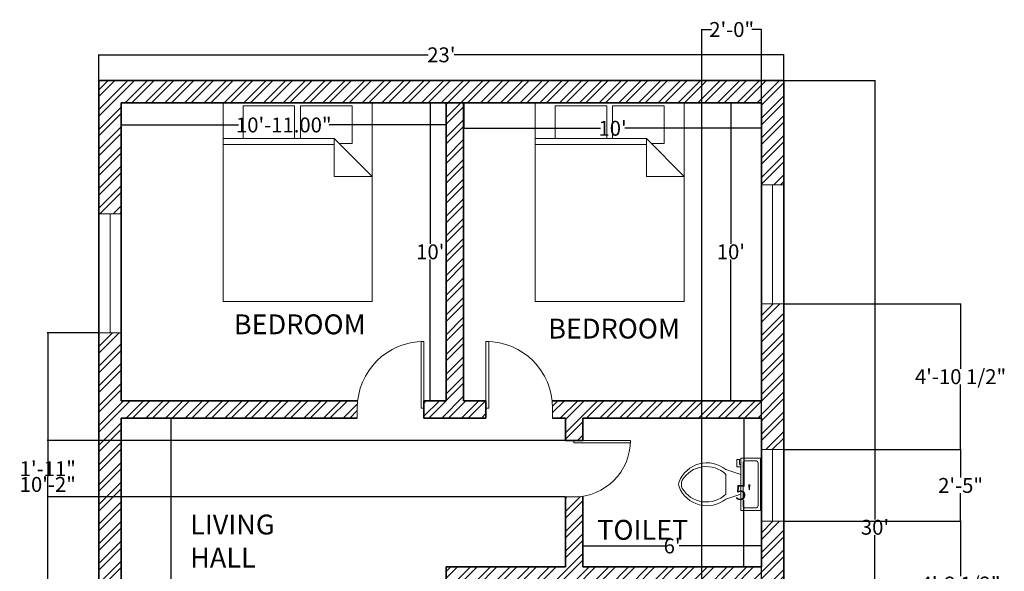
# Model space of a CAD drawing. Units: inches. Extents: x -20 to 887, y -143 to 410.
# Tile 3 of 5: x -15 to 381, y 180 to 403. Entities that reach past the tile are written whole.
import ezdxf

# ---------------------------------------------------------------- set-up
doc = ezdxf.new("R2010")
doc.units = ezdxf.units.IN
doc.header["$MEASUREMENT"] = 0
for name, color, linetype, lineweight in [('A-ANNO-DIMS', 2, 'Continuous', 18), ('A-AREA-IDEN', 7, 'Continuous', 25), ('A-DOOR', 3, 'Continuous', 18), ('A-FLOR-FIXT', 9, 'Continuous', 18), ('A-FURN', 8, 'Continuous', 18), ('A-GLAZ', 4, 'Continuous', 18), ('A-WALL', 7, 'Continuous', 35), ('A-WALL-PATT', 8, 'Continuous', 13)]:
    doc.layers.add(name, color=color, linetype=linetype, lineweight=lineweight)
doc.styles.get("Standard").update_dxf_attribs({"font": 'arial.ttf'})
doc.dimstyles.get("Standard").update_dxf_attribs({"dimtxt": 6, "dimasz": 0.18, "dimexe": 0.18, "dimexo": 0.0625, "dimgap": 0.09, "dimtad": 0, "dimtih": 1, "dimtoh": 1, "dimzin": 0, "dimdsep": 46, "dimlunit": 3, "dimtxsty": 'Standard', "dimcen": 0.09, "dimadec": 0, "dimazin": 0, "dimtfac": 1, "dimtofl": 0, "dimtmove": 0, "dimatfit": 3, "dimfxl": 1, "dimtolj": 1, "dimtzin": 0, "dimarcsym": 0})

# ---------------------------------------------------------------- blocks, each defined once
blk = doc.blocks.new('*U2')
for p, q in [((0, 0), (0, -6)), ((40, 0), (40, -6))]:
    blk.add_line(p, q)
blk.add_lwpolyline([(0, 0), (0, 40), (1.75, 40), (1.75, 0)], close=True)
blk.add_arc((0, 0), 40, 0, 90)
blk = doc.blocks.new('*U6')
for p, q in [((9.5, -6), (9.5, -2)), ((-10, -8.5), (-8, -8.5)), ((-10, -9.5), (-10, -8.5)), ((-7, -9.5), (-10, -9.5)), ((-8, -8.5), (-8, -8)), ((-7, -8), (-7, -9.5)), ((-4, -8), (-6, -14)), ((4, -8), (6, -14)), ((4, -14), (-4, -14))]:
    blk.add_line(p, q)
blk.add_lwpolyline([(10.5, -8), (10.5, 0), (-10.5, 0), (-10.5, -8)], close=True)
for points in [[(-9.5, -2), (-9.5, -6)], [(8.5, -1), (-8.5, -1)], [(-8.5, -7), (8.5, -7)]]:
    blk.add_lwpolyline(points)
for centre, radius, start, end in [((-8.62, -1.88), 0.884, 81.8699, 188.1301), ((8.62, -1.88), 0.884, 351.8699, 98.1301), ((-8.62, -6.12), 0.884, 171.8699, 278.1301), ((8.62, -6.12), 0.884, 261.8699, 8.1301), ((3.52, -21.58), 12.17, 141.4691, 247.9714), ((4.2, -21.82), 11.33, 136.3677, 238.9468), ((-3.52, -21.58), 12.17, 292.0284, 38.5307), ((-4.2, -21.82), 11.33, 301.053, 43.6321), ((0, -27.88), 4, 245.7318, 294.2682), ((0, -29), 4, 254.8605, 285.1395)]:
    blk.add_arc(centre, radius, start, end)
blk = doc.blocks.new('Bed - Queen')
for p, q in [((0, -80.00003), (0, 0)), ((0, 0), (59.99999, 0)), ((59.99999, 0), (59.99999, -80.00003)), ((7.99999, -1.2), (28.79998, -1.2)), ((7.99999, -14.4), (7.99999, -1.2)), ((28.79998, -1.2), (28.79998, -14.4)), ((31.19999, -1.2), (51.99999, -1.2)), ((31.19999, -14.4), (31.19999, -1.2)), ((51.99999, -1.2), (51.99999, -16.4)), ((0, -14.4), (44.8, -14.4)), ((59.99999, -29.6), (44.8, -14.4)), ((44.8, -14.4), (44.8, -29.6)), ((44.8, -16.8), (0, -16.8)), ((51.99999, -16.4), (46.79936, -16.4)), ((44.8, -29.6), (59.99999, -29.6)), ((59.99999, -80.00003), (0, -80.00003))]:
    blk.add_line(p, q)
blk = doc.blocks.new('*D11')
at = {"layer": 'A-ANNO-DIMS', "color": 0, "lineweight": -2, "transparency": 16777216}
for p, q in [((25.48, 242.13), (45.6, 242.13)), ((45.42, 241.95), (45.42, 137.79)), ((45.42, 27.31), (45.42, 131.48)), ((25.48, 27.13), (45.6, 27.13))]:
    blk.add_line(p, q, dxfattribs=at)
at = {"layer": 'A-ANNO-DIMS', "color": 0, "transparency": 16777216}
for points in [[(45.39, 241.95), (45.45, 241.95), (45.42, 242.13)], [(45.39, 27.31), (45.45, 27.31), (45.42, 27.13)]]:
    blk.add_solid(points, dxfattribs=at)
at = {"layer": 'Defpoints', "color": 0, "transparency": 16777216}
for p in [(25.42, 242.13), (25.42, 27.13), (45.42, 27.13)]:
    blk.add_point(p, dxfattribs=at)
at = {"layer": 'A-ANNO-DIMS', "color": 0, "transparency": 16777216, "insert": (45.42, 134.63), "char_height": 6, "attachment_point": 5}
blk.add_mtext('\\A1;17\'-11.00"', dxfattribs=at)
blk = doc.blocks.new('*D15')
at = {"layer": 'A-ANNO-DIMS', "color": 0, "lineweight": -2, "transparency": 16777216}
for p, q in [((283.35, 242.13), (276.08, 242.13)), ((276.26, 241.95), (276.26, 215.28)), ((276.26, 182.31), (276.26, 208.99)), ((283.35, 182.13), (276.08, 182.13))]:
    blk.add_line(p, q, dxfattribs=at)
at = {"layer": 'A-ANNO-DIMS', "color": 0, "transparency": 16777216}
for points in [[(276.23, 241.95), (276.29, 241.95), (276.26, 242.13)], [(276.23, 182.31), (276.29, 182.31), (276.26, 182.13)]]:
    blk.add_solid(points, dxfattribs=at)
at = {"layer": 'Defpoints', "color": 0, "transparency": 16777216}
for p in [(276.26, 242.13), (283.42, 242.13), (283.42, 182.13)]:
    blk.add_point(p, dxfattribs=at)
at = {"layer": 'A-ANNO-DIMS', "color": 0, "transparency": 16777216, "insert": (276.26, 212.13), "char_height": 6, "attachment_point": 5}
blk.add_mtext("\\A1;5'", dxfattribs=at)
blk = doc.blocks.new('*D16')
at = {"layer": 'A-ANNO-DIMS', "color": 0, "lineweight": -2, "transparency": 16777216}
for p, q in [((211.42, 182.2), (211.42, 190.79)), ((211.6, 190.61), (244.55, 190.61)), ((283.24, 190.61), (250.28, 190.61)), ((283.42, 182.2), (283.42, 190.79))]:
    blk.add_line(p, q, dxfattribs=at)
at = {"layer": 'A-ANNO-DIMS', "color": 0, "transparency": 16777216}
for points in [[(211.6, 190.64), (211.6, 190.58), (211.42, 190.61)], [(283.24, 190.64), (283.24, 190.58), (283.42, 190.61)]]:
    blk.add_solid(points, dxfattribs=at)
at = {"layer": 'Defpoints', "color": 0, "transparency": 16777216}
for p in [(283.42, 190.61), (211.42, 182.13), (283.42, 182.13)]:
    blk.add_point(p, dxfattribs=at)
at = {"layer": 'A-ANNO-DIMS', "color": 0, "transparency": 16777216, "insert": (247.42, 190.61), "char_height": 6, "attachment_point": 5}
blk.add_mtext("\\A1;6'", dxfattribs=at)
blk = doc.blocks.new('*D17')
at = {"layer": 'A-ANNO-DIMS', "color": 0, "lineweight": -2, "transparency": 16777216}
for p, q in [((283.35, 369.13), (270.92, 369.13)), ((271.1, 368.95), (271.1, 312.29)), ((271.1, 249.31), (271.1, 305.98)), ((283.35, 249.13), (270.92, 249.13))]:
    blk.add_line(p, q, dxfattribs=at)
at = {"layer": 'A-ANNO-DIMS', "color": 0, "transparency": 16777216}
for points in [[(271.07, 368.95), (271.13, 368.95), (271.1, 369.13)], [(271.07, 249.31), (271.13, 249.31), (271.1, 249.13)]]:
    blk.add_solid(points, dxfattribs=at)
at = {"layer": 'Defpoints', "color": 0, "transparency": 16777216}
for p in [(271.1, 369.13), (283.42, 369.13), (283.42, 249.13)]:
    blk.add_point(p, dxfattribs=at)
at = {"layer": 'A-ANNO-DIMS', "color": 0, "transparency": 16777216, "insert": (271.1, 309.13), "char_height": 6, "attachment_point": 5}
blk.add_mtext("\\A1;10'", dxfattribs=at)
blk = doc.blocks.new('*D18')
at = {"layer": 'A-ANNO-DIMS', "color": 0, "lineweight": -2, "transparency": 16777216}
for p, q in [((163.42, 369.07), (163.42, 358.72)), ((283.42, 369.07), (283.42, 358.72)), ((163.6, 358.9), (218.52, 358.9)), ((283.24, 358.9), (228.32, 358.9))]:
    blk.add_line(p, q, dxfattribs=at)
at = {"layer": 'A-ANNO-DIMS', "color": 0, "transparency": 16777216}
for points in [[(163.6, 358.93), (163.6, 358.87), (163.42, 358.9)], [(283.24, 358.93), (283.24, 358.87), (283.42, 358.9)]]:
    blk.add_solid(points, dxfattribs=at)
at = {"layer": 'Defpoints', "color": 0, "transparency": 16777216}
for p in [(163.42, 369.13), (283.42, 369.13), (283.42, 358.9)]:
    blk.add_point(p, dxfattribs=at)
at = {"layer": 'A-ANNO-DIMS', "color": 0, "transparency": 16777216, "insert": (223.42, 358.9), "char_height": 6, "attachment_point": 5}
blk.add_mtext("\\A1;10'", dxfattribs=at)
blk = doc.blocks.new('*D19')
at = {"layer": 'A-ANNO-DIMS', "color": 0, "lineweight": -2, "transparency": 16777216}
for p, q in [((156.35, 369.13), (149.78, 369.13)), ((149.96, 368.95), (149.96, 312.29)), ((149.96, 249.31), (149.96, 305.98)), ((156.35, 249.13), (149.78, 249.13))]:
    blk.add_line(p, q, dxfattribs=at)
at = {"layer": 'A-ANNO-DIMS', "color": 0, "transparency": 16777216}
for points in [[(149.93, 368.95), (149.99, 368.95), (149.96, 369.13)], [(149.93, 249.31), (149.99, 249.31), (149.96, 249.13)]]:
    blk.add_solid(points, dxfattribs=at)
at = {"layer": 'Defpoints', "color": 0, "transparency": 16777216}
for p in [(149.96, 369.13), (156.42, 369.13), (156.42, 249.13)]:
    blk.add_point(p, dxfattribs=at)
at = {"layer": 'A-ANNO-DIMS', "color": 0, "transparency": 16777216, "insert": (149.96, 309.13), "char_height": 6, "attachment_point": 5}
blk.add_mtext("\\A1;10'", dxfattribs=at)
blk = doc.blocks.new('*D20')
at = {"layer": 'A-ANNO-DIMS', "color": 0, "lineweight": -2, "transparency": 16777216}
for p, q in [((25.42, 369.07), (25.42, 360.07)), ((156.42, 369.07), (156.42, 360.07)), ((25.6, 360.25), (72.65, 360.25)), ((156.24, 360.25), (109.19, 360.25))]:
    blk.add_line(p, q, dxfattribs=at)
at = {"layer": 'A-ANNO-DIMS', "color": 0, "transparency": 16777216}
for points in [[(25.6, 360.28), (25.6, 360.22), (25.42, 360.25)], [(156.24, 360.28), (156.24, 360.22), (156.42, 360.25)]]:
    blk.add_solid(points, dxfattribs=at)
at = {"layer": 'Defpoints', "color": 0, "transparency": 16777216}
for p in [(25.42, 369.13), (156.42, 369.13), (156.42, 360.25)]:
    blk.add_point(p, dxfattribs=at)
at = {"layer": 'A-ANNO-DIMS', "color": 0, "transparency": 16777216, "insert": (90.92, 360.25), "char_height": 6, "attachment_point": 5}
blk.add_mtext('\\A1;10\'-11.00"', dxfattribs=at)
blk = doc.blocks.new('*D21')
at = {"layer": 'A-ANNO-DIMS', "color": 0, "lineweight": -2, "transparency": 16777216}
for p, q in [((16.42, 378.2), (16.42, 388.69)), ((16.6, 388.51), (149.18, 388.51)), ((292.24, 388.51), (159.65, 388.51)), ((292.42, 378.2), (292.42, 388.69))]:
    blk.add_line(p, q, dxfattribs=at)
at = {"layer": 'A-ANNO-DIMS', "color": 0, "transparency": 16777216}
for points in [[(16.6, 388.54), (16.6, 388.48), (16.42, 388.51)], [(292.24, 388.54), (292.24, 388.48), (292.42, 388.51)]]:
    blk.add_solid(points, dxfattribs=at)
at = {"layer": 'Defpoints', "color": 0, "transparency": 16777216}
for p in [(292.42, 388.51), (16.42, 378.13), (292.42, 378.13)]:
    blk.add_point(p, dxfattribs=at)
at = {"layer": 'A-ANNO-DIMS', "color": 0, "transparency": 16777216, "insert": (154.42, 388.51), "char_height": 6, "attachment_point": 5}
blk.add_mtext("\\A1;23'", dxfattribs=at)
blk = doc.blocks.new('*D22')
at = {"layer": 'A-ANNO-DIMS', "color": 0, "lineweight": -2, "transparency": 16777216}
for p, q in [((292.48, 378.13), (329.35, 378.13)), ((329.17, 377.95), (329.17, 201.29)), ((329.17, 18.31), (329.17, 194.98)), ((292.48, 18.13), (329.35, 18.13))]:
    blk.add_line(p, q, dxfattribs=at)
at = {"layer": 'A-ANNO-DIMS', "color": 0, "transparency": 16777216}
for points in [[(329.14, 377.95), (329.2, 377.95), (329.17, 378.13)], [(329.14, 18.31), (329.2, 18.31), (329.17, 18.13)]]:
    blk.add_solid(points, dxfattribs=at)
at = {"layer": 'Defpoints', "color": 0, "transparency": 16777216}
for p in [(292.42, 378.13), (292.42, 18.13), (329.17, 18.13)]:
    blk.add_point(p, dxfattribs=at)
at = {"layer": 'A-ANNO-DIMS', "color": 0, "transparency": 16777216, "insert": (329.17, 198.13), "char_height": 6, "attachment_point": 5}
blk.add_mtext("\\A1;30'", dxfattribs=at)
blk = doc.blocks.new('WIN-48IN-9IN-WALL')
for p, q in [((9, 48), (0, 48)), ((4.5, 0), (4.5, 48)), ((9, 0), (0, 0))]:
    blk.add_line(p, q)
blk = doc.blocks.new('*D60')
at = {"layer": 'A-ANNO-DIMS', "color": 0, "lineweight": -2, "transparency": 16777216}
for p, q in [((16.35, 276.44), (-4.36, 276.44)), ((-4.18, 276.26), (-4.18, 218.55)), ((-4.18, 154.54), (-4.18, 212.25)), ((16.35, 154.36), (-4.36, 154.36))]:
    blk.add_line(p, q, dxfattribs=at)
at = {"layer": 'A-ANNO-DIMS', "color": 0, "transparency": 16777216}
for points in [[(-4.21, 276.26), (-4.15, 276.26), (-4.18, 276.44)], [(-4.21, 154.54), (-4.15, 154.54), (-4.18, 154.36)]]:
    blk.add_solid(points, dxfattribs=at)
at = {"layer": 'Defpoints', "color": 0, "transparency": 16777216}
for p in [(-4.18, 276.44), (16.42, 276.44), (16.42, 154.36)]:
    blk.add_point(p, dxfattribs=at)
at = {"layer": 'A-ANNO-DIMS', "color": 0, "transparency": 16777216, "insert": (-4.18, 215.4), "char_height": 6, "attachment_point": 5}
blk.add_mtext('\\A1;10\'-2"', dxfattribs=at)
blk = doc.blocks.new('*D63')
at = {"layer": 'A-ANNO-DIMS', "color": 0, "lineweight": -2, "transparency": 16777216}
for p, q in [((292.48, 200.53), (363.84, 200.53)), ((363.66, 200.35), (363.66, 178.43)), ((363.66, 150.12), (363.66, 172.04)), ((292.48, 149.94), (363.84, 149.94))]:
    blk.add_line(p, q, dxfattribs=at)
at = {"layer": 'A-ANNO-DIMS', "color": 0, "transparency": 16777216}
for points in [[(363.63, 200.35), (363.69, 200.35), (363.66, 200.53)], [(363.63, 150.12), (363.69, 150.12), (363.66, 149.94)]]:
    blk.add_solid(points, dxfattribs=at)
at = {"layer": 'Defpoints', "color": 0, "transparency": 16777216}
for p in [(292.42, 200.53), (363.66, 200.53), (292.42, 149.94)]:
    blk.add_point(p, dxfattribs=at)
at = {"layer": 'A-ANNO-DIMS', "color": 0, "transparency": 16777216, "insert": (363.66, 175.23), "char_height": 6, "attachment_point": 5}
blk.add_mtext('\\A1;4\'-2 1/2"', dxfattribs=at)
blk = doc.blocks.new('*D64')
at = {"layer": 'A-ANNO-DIMS', "color": 0, "lineweight": -2, "transparency": 16777216}
for p, q in [((292.48, 229.46), (363.84, 229.46)), ((363.66, 229.28), (363.66, 218.15)), ((363.66, 200.71), (363.66, 211.84)), ((292.48, 200.53), (363.84, 200.53))]:
    blk.add_line(p, q, dxfattribs=at)
at = {"layer": 'A-ANNO-DIMS', "color": 0, "transparency": 16777216}
for points in [[(363.63, 229.28), (363.69, 229.28), (363.66, 229.46)], [(363.63, 200.71), (363.69, 200.71), (363.66, 200.53)]]:
    blk.add_solid(points, dxfattribs=at)
at = {"layer": 'Defpoints', "color": 0, "transparency": 16777216}
for p in [(292.42, 229.46), (363.66, 229.46), (292.42, 200.53)]:
    blk.add_point(p, dxfattribs=at)
at = {"layer": 'A-ANNO-DIMS', "color": 0, "transparency": 16777216, "insert": (363.66, 214.99), "char_height": 6, "attachment_point": 5}
blk.add_mtext('\\A1;2\'-5"', dxfattribs=at)
blk = doc.blocks.new('*D65')
at = {"layer": 'A-ANNO-DIMS', "color": 0, "lineweight": -2, "transparency": 16777216}
for p, q in [((292.48, 288.18), (363.84, 288.18)), ((363.66, 288), (363.66, 262.01)), ((363.66, 229.64), (363.66, 255.63)), ((292.48, 229.46), (363.84, 229.46))]:
    blk.add_line(p, q, dxfattribs=at)
at = {"layer": 'A-ANNO-DIMS', "color": 0, "transparency": 16777216}
for points in [[(363.63, 288), (363.69, 288), (363.66, 288.18)], [(363.63, 229.64), (363.69, 229.64), (363.66, 229.46)]]:
    blk.add_solid(points, dxfattribs=at)
at = {"layer": 'Defpoints', "color": 0, "transparency": 16777216}
for p in [(292.42, 288.18), (363.66, 288.18), (292.42, 229.46)]:
    blk.add_point(p, dxfattribs=at)
at = {"layer": 'A-ANNO-DIMS', "color": 0, "transparency": 16777216, "insert": (363.66, 258.82), "char_height": 6, "attachment_point": 5}
blk.add_mtext('\\A1;4\'-10 1/2"', dxfattribs=at)
blk = doc.blocks.new('*D70')
at = {"layer": 'A-ANNO-DIMS', "color": 0, "lineweight": -2, "transparency": 16777216}
for p, q in [((259.42, 27.2), (259.42, 398.91)), ((259.6, 398.73), (263.3, 398.73)), ((283.24, 398.73), (279.53, 398.73)), ((283.42, 27.2), (283.42, 398.91))]:
    blk.add_line(p, q, dxfattribs=at)
at = {"layer": 'A-ANNO-DIMS', "color": 0, "transparency": 16777216}
for points in [[(259.6, 398.76), (259.6, 398.7), (259.42, 398.73)], [(283.24, 398.76), (283.24, 398.7), (283.42, 398.73)]]:
    blk.add_solid(points, dxfattribs=at)
at = {"layer": 'Defpoints', "color": 0, "transparency": 16777216}
for p in [(283.42, 398.73), (259.42, 27.13), (283.42, 27.13)]:
    blk.add_point(p, dxfattribs=at)
at = {"layer": 'A-ANNO-DIMS', "color": 0, "transparency": 16777216, "insert": (271.42, 398.73), "char_height": 6, "attachment_point": 5}
blk.add_mtext('\\A1;2\'-0"', dxfattribs=at)
blk = doc.blocks.new('*D71')
at = {"layer": 'A-ANNO-DIMS', "color": 0, "lineweight": -2, "transparency": 16777216}
for p, q in [((204.35, 233.13), (-4.36, 233.13)), ((-4.18, 232.95), (-4.18, 224.83)), ((-4.18, 210.51), (-4.18, 218.63)), ((204.35, 210.33), (-4.36, 210.33))]:
    blk.add_line(p, q, dxfattribs=at)
at = {"layer": 'A-ANNO-DIMS', "color": 0, "transparency": 16777216}
for points in [[(-4.21, 232.95), (-4.15, 232.95), (-4.18, 233.13)], [(-4.21, 210.51), (-4.15, 210.51), (-4.18, 210.33)]]:
    blk.add_solid(points, dxfattribs=at)
at = {"layer": 'Defpoints', "color": 0, "transparency": 16777216}
for p in [(-4.18, 233.13), (204.42, 233.13), (204.42, 210.33)]:
    blk.add_point(p, dxfattribs=at)
at = {"layer": 'A-ANNO-DIMS', "color": 0, "transparency": 16777216, "insert": (-4.18, 221.73), "char_height": 6, "attachment_point": 5}
blk.add_mtext('\\A1;1\'-11"', dxfattribs=at)

msp = doc.modelspace()

# ---------------------------------------------------------------- hatches: boundary and pattern name
at = {"layer": 'A-WALL-PATT'}
h = msp.add_hatch(dxfattribs=at)
h.set_pattern_fill('ANSI32', color=256, scale=15)
h.paths.add_polyline_path([(25.417, 369.135), (26.83, 369.135), (283.417, 369.135), (283.417, 336.183), (292.417, 336.183), (292.417, 378.135), (16.417, 378.135), (16.417, 324.435), (25.417, 324.435)])
h = msp.add_hatch(dxfattribs=at)
h.set_pattern_fill('ANSI32', color=256, scale=15)
h.paths.add_polyline_path([(163.417, 369.135), (156.417, 369.135), (156.417, 249.135), (147.417, 249.135), (147.417, 246.163), (147.417, 242.135), (172.417, 242.135), (172.417, 246.163), (172.417, 249.135), (163.417, 249.135)])
h = msp.add_hatch(dxfattribs=at)
h.set_pattern_fill('ANSI32', color=256, scale=15)
h.paths.add_polyline_path([(292.417, 288.183), (283.417, 288.183), (283.417, 249.135), (199.107, 249.135, -0.0277279), (199.272, 246.163), (199.272, 242.135), (204.417, 242.135), (204.417, 233.135), (207.838, 233.135), (211.417, 233.135), (211.417, 242.135), (283.417, 242.135), (283.417, 229.456), (292.417, 229.456)])
h = msp.add_hatch(dxfattribs=at)
h.set_pattern_fill('ANSI32', color=256, scale=15)
h.paths.add_polyline_path([(25.417, 242.135), (120.561, 242.135), (120.561, 246.163, -0.0277279), (120.726, 249.135), (25.417, 249.135), (25.417, 276.435), (16.417, 276.435), (16.417, 154.363), (25.417, 154.363)])
h = msp.add_hatch(dxfattribs=at)
h.set_pattern_fill('ANSI32', color=256, scale=15)
h.paths.add_polyline_path([(292.417, 200.529), (283.417, 200.529), (283.417, 182.135), (211.417, 182.135), (211.417, 210.612, -0.0394206), (207.838, 210.33), (204.417, 210.33), (204.417, 182.135), (156.417, 182.135), (156.417, 154.102), (163.417, 154.102), (163.417, 174.135), (283.417, 174.135), (283.417, 149.94), (292.417, 149.94)])

# ---------------------------------------------------------------- linework, layer by layer
at = {"layer": 'A-GLAZ'}
for p, q in [((283.417, 336.183), (292.417, 336.183)), ((287.917, 288.183), (287.879, 336.183)), ((283.417, 288.183), (292.417, 288.183)), ((283.417, 229.456), (292.417, 229.456)), ((287.917, 200.529), (287.917, 229.456)), ((283.417, 200.529), (292.417, 200.529))]:
    msp.add_line(p, q, dxfattribs=at)
at = {"layer": 'A-WALL'}
msp.add_lwpolyline([(16.417, 18.135), (292.417, 18.135), (292.417, 378.135), (16.417, 378.135)], close=True, dxfattribs=at)
for points in [[(26.83, 369.135), (25.417, 369.135), (25.417, 249.135)], [(283.417, 369.135), (26.83, 369.135)], [(156.417, 369.135), (156.417, 249.135)], [(163.417, 249.135), (163.417, 369.135)], [(283.417, 249.135), (283.417, 369.135)], [(120.726, 249.135), (25.417, 249.135)], [(147.417, 249.135), (147.417, 242.135)], [(156.417, 249.135), (147.417, 249.135)], [(172.417, 249.135), (163.417, 249.135)], [(172.417, 242.135), (172.417, 249.135)], [(283.417, 249.135), (199.107, 249.135)], [(120.561, 242.135), (25.417, 242.135)], [(25.417, 242.135), (25.417, 27.135)], [(172.417, 242.135), (147.417, 242.135)], [(204.417, 242.135), (199.272, 242.135)], [(204.417, 233.135), (204.417, 242.135)], [(283.417, 242.135), (211.417, 242.135)], [(211.417, 233.135), (211.417, 242.135)], [(283.417, 182.135), (283.417, 242.135)], [(211.417, 233.135), (204.417, 233.135)], [(204.417, 182.135), (204.417, 210.33)], [(211.417, 182.135), (211.417, 210.612)], [(156.417, 182.135), (204.417, 182.135)], [(156.417, 182.135), (156.417, 154.102)], [(211.417, 182.135), (283.417, 182.135)]]:
    msp.add_lwpolyline(points, dxfattribs=at)

# ---------------------------------------------------------------- block references
at = {"layer": 'A-DOOR', "yscale": 0.6713823920216754, "zscale": 0.6713823920216754}
for p, xscale in [((147.417, 246.163), -0.6713823920216754), ((172.417, 246.163), 0.6713823920216754)]:
    msp.add_blockref('*U2', p, dxfattribs=dict(at, xscale=xscale))
at = {"layer": 'A-DOOR', "xscale": 0.570126991445634, "yscale": 0.570126991445634, "zscale": 0.570126991445634, "rotation": 270}
msp.add_blockref('*U2', (207.838, 233.135), dxfattribs=at)
at = {"layer": 'A-FLOR-FIXT', "rotation": 270}
msp.add_blockref('*U6', (283.057, 215.448), dxfattribs=at)
at = {"layer": 'A-FURN'}
for p in [(66.498, 369.135), (192.26, 369.135)]:
    msp.add_blockref('Bed - Queen', p, dxfattribs=at)
at = {"layer": 'A-GLAZ'}
msp.add_blockref('WIN-48IN-9IN-WALL', (16.417, 276.435), dxfattribs=at)

# ---------------------------------------------------------------- texts
at = {"layer": 'A-AREA-IDEN', "char_height": 8, "attachment_point": 1}
for s, insert in [('BEDROOM', (70.793, 283.908)), ('BEDROOM', (197.475, 282.191)), ('LIVING HALL', (53.186, 203.231)), ('TOILET', (217.229, 201.086))]:
    msp.add_mtext_dynamic_manual_height_columns(s, width=50.36765, gutter_width=1, heights=[0], dxfattribs=dict(at, insert=insert))

# ---------------------------------------------------------------- dimensions: what is measured, and where the dimension line sits
at = {"layer": 'A-ANNO-DIMS'}
for base, p1, p2, override, picture, middle in [((283.417, 398.735), (259.417, 27.135), (283.417, 27.135), {"dimdec": 1, "dimlfac": 1, "dimrnd": 0, "dimzin": 1, "dimdsep": 46, "dimlunit": 4, "dimfrac": 2}, '*D70', (271.417, 398.735)), ((292.417, 388.511), (16.417, 378.135), (292.417, 378.135), {"dimclrd": 0, "dimclre": 0, "dimclrt": 0}, '*D21', (154.417, 388.511)), ((156.417, 360.246), (25.417, 369.135), (156.417, 369.135), {"dimclrd": 0, "dimclre": 0, "dimclrt": 0}, '*D20', (90.917, 360.246)), ((283.417, 358.9), (163.417, 369.135), (283.417, 369.135), {"dimclrd": 0, "dimclre": 0, "dimclrt": 0}, '*D18', (223.417, 358.9)), ((283.417, 190.609), (211.417, 182.135), (283.417, 182.135), {"dimclrd": 0, "dimclre": 0, "dimclrt": 0}, '*D16', (247.417, 190.609))]:
    dim = msp.add_linear_dim(base=base, p1=p1, p2=p2, dimstyle='Standard', override=override, dxfattribs=at)
    dim.commit()
    dim.dimension.update_dxf_attribs({"geometry": picture, "text_midpoint": middle})
for base, p1, p2, override, picture, middle in [((329.167, 18.135), (292.417, 378.135), (292.417, 18.135), {"dimclrd": 0, "dimclre": 0, "dimclrt": 0}, '*D22', (329.167, 198.135)), ((149.96, 369.135), (156.417, 249.135), (156.417, 369.135), {"dimclrd": 0, "dimclre": 0, "dimclrt": 0}, '*D19', (149.96, 309.135)), ((271.097, 369.135), (283.417, 249.135), (283.417, 369.135), {"dimclrd": 0, "dimclre": 0, "dimclrt": 0}, '*D17', (271.097, 309.135)), ((363.657, 288.183), (292.417, 229.456), (292.417, 288.183), {"dimdec": 1, "dimlfac": 1, "dimrnd": 0, "dimzin": 1, "dimdsep": 46, "dimlunit": 4, "dimfrac": 2}, '*D65', (363.657, 258.82)), ((-4.183, 276.435), (16.417, 154.363), (16.417, 276.435), {"dimdec": 1, "dimlfac": 1, "dimrnd": 0, "dimzin": 1, "dimdsep": 46, "dimlunit": 4, "dimfrac": 2}, '*D60', (-4.183, 215.399)), ((45.415, 27.135), (25.417, 242.135), (25.417, 27.135), {"dimclrd": 0, "dimclre": 0, "dimclrt": 0}, '*D11', (45.415, 134.635)), ((276.265, 242.135), (283.417, 182.135), (283.417, 242.135), {"dimclrd": 0, "dimclre": 0, "dimclrt": 0}, '*D15', (276.265, 212.135)), ((-4.183, 233.135), (204.417, 210.33), (204.417, 233.135), {"dimdec": 1, "dimlfac": 1, "dimrnd": 0, "dimzin": 1, "dimdsep": 46, "dimlunit": 4, "dimfrac": 2}, '*D71', (-4.183, 221.732)), ((363.657, 229.456), (292.417, 200.529), (292.417, 229.456), {"dimdec": 1, "dimlfac": 1, "dimrnd": 0, "dimzin": 1, "dimdsep": 46, "dimlunit": 4, "dimfrac": 2}, '*D64', (363.657, 214.993)), ((363.657, 200.529), (292.417, 149.94), (292.417, 200.529), {"dimdec": 1, "dimlfac": 1, "dimrnd": 0, "dimzin": 1, "dimdsep": 46, "dimlunit": 4, "dimfrac": 2}, '*D63', (363.657, 175.234))]:
    dim = msp.add_linear_dim(base=base, p1=p1, p2=p2, angle=90, dimstyle='Standard', override=override, dxfattribs=at)
    dim.commit()
    dim.dimension.update_dxf_attribs({"geometry": picture, "text_midpoint": middle})

doc.saveas('drawing.dxf')
